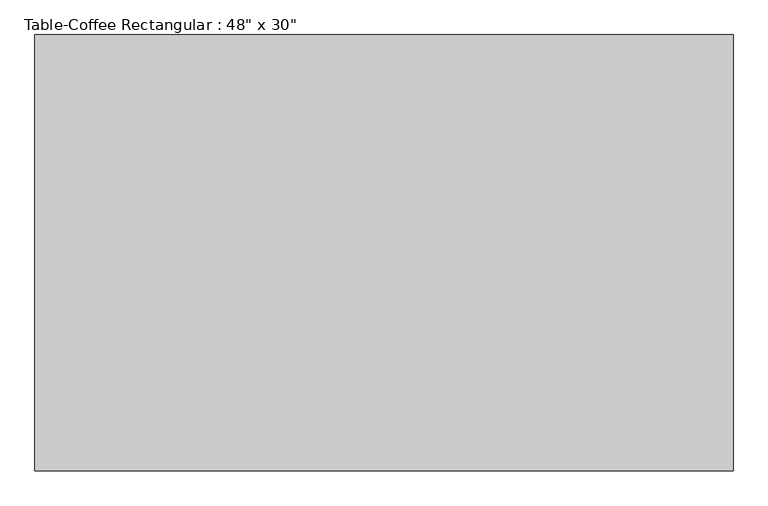
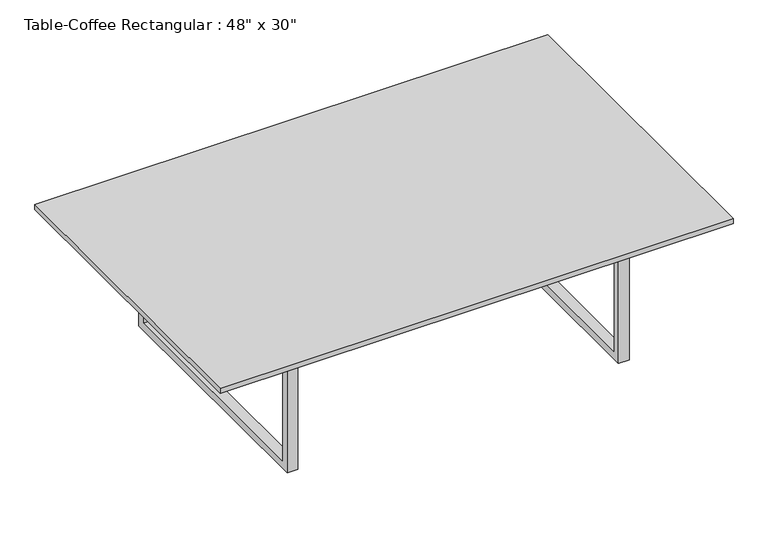
"""IFC4 building model written with IfcOpenShell, lengths in millimetres: furniture geometry."""

from ifc_helpers import new_model, si_unit, frame, origin, place, context, project, spatial, polyline, outline, extrude, source, transform, mapped, element, save


def furniture_acc2807d(model_context):
    return source(origin(), model_context, "Body", "SweptSolid", [
        extrude(outline(polyline([(1222.9336303, 750.6108318), (1222.9336303, -11.3891682), (3.7336303, -11.3891682), (3.7336303, 750.6108318), (1222.9336303, 750.6108318)])), frame((0.0, 0.0, 317.5), z_axis=(0.0, 0.0, 1.0), x_axis=(1.0, 0.0, 0.0)), (0.0, 0.0, 1.0), 12.7),
        extrude(outline(polyline([(64.8108318, 317.5), (674.4108318, 317.5), (674.4108318, 0.0), (64.8108318, 0.0), (64.8108318, 317.5)]), holes=[polyline([(83.8608318, 298.45), (83.8608318, 19.05), (655.3608318, 19.05), (655.3608318, 298.45), (83.8608318, 298.45)])]), frame((206.9336303, 0.0, 0.0), z_axis=(1.0, 0.0, 0.0), x_axis=(0.0, 1.0, 0.0)), (0.0, 0.0, 1.0), 25.4),
        extrude(outline(polyline([(64.8108318, 317.5), (674.4108318, 317.5), (674.4108318, 0.0), (64.8108318, 0.0), (64.8108318, 317.5)]), holes=[polyline([(83.8608318, 298.45), (83.8608318, 19.05), (655.3608318, 19.05), (655.3608318, 298.45), (83.8608318, 298.45)])]), frame((994.3336303, 0.0, 0.0), z_axis=(1.0, 0.0, 0.0), x_axis=(0.0, 1.0, 0.0)), (0.0, 0.0, 1.0), 25.4),
        extrude(outline(polyline([(994.3336303, 379.1358318), (994.3336303, 360.0858318), (232.3336303, 360.0858318), (232.3336303, 379.1358318), (994.3336303, 379.1358318)])), frame((0.0, 0.0, 298.45), z_axis=(0.0, 0.0, 1.0), x_axis=(1.0, 0.0, 0.0)), (0.0, 0.0, 1.0), 19.05),
    ])


if __name__ == "__main__":
    model = new_model("IFC4")
    model_context = context("Model", 3, world=origin())
    ifc_project = project(units=[si_unit("LENGTHUNIT", "METRE", prefix="MILLI")], contexts=[model_context])
    site = spatial("IfcSite", under=ifc_project)
    building = spatial("IfcBuilding", under=site)
    placement = place(None, origin())
    furniture_shape = furniture_acc2807d(model_context)
    element("IfcFurniture", 1, ObjectType="Table-Coffee Rectangular : 48\" x 30\"", at=placement, inside=building, context=model_context, shape_type="MappedRepresentation", body=[
        mapped(furniture_shape, transform((0.0, 0.0, 0.0), x_axis=(1.0, 0.0, 0.0), y_axis=(0.0, 1.0, 0.0), z_axis=(0.0, 0.0, 1.0))),
    ])
    save(model, "model.ifc")

# Revit data of these elements
# Type "Table-Coffee Rectangular : 48\" x 30\""
#   Assembly Code = "E2020200"
#   Height = 1.083333 ft
#   Length = 4 ft
#   Width = 2.5 ft
#   Base Material = Metal - Chrome
#   Table Top Material = Glass - Clear, Grey
#   Default Elevation = 0
# Element 1 (IfcFurniture, "Table-Coffee Rectangular : 48\" x 30\"")
#   Materials on its faces: "Metal - Chrome", "Glass - Clear, Grey"
# Materials
#   "Metal - Chrome": class "Metal", colour RGB 247 247 247, transparency 0
#   "Glass - Clear, Grey": class "Glass", colour RGB 252 255 255, transparency 0.64
